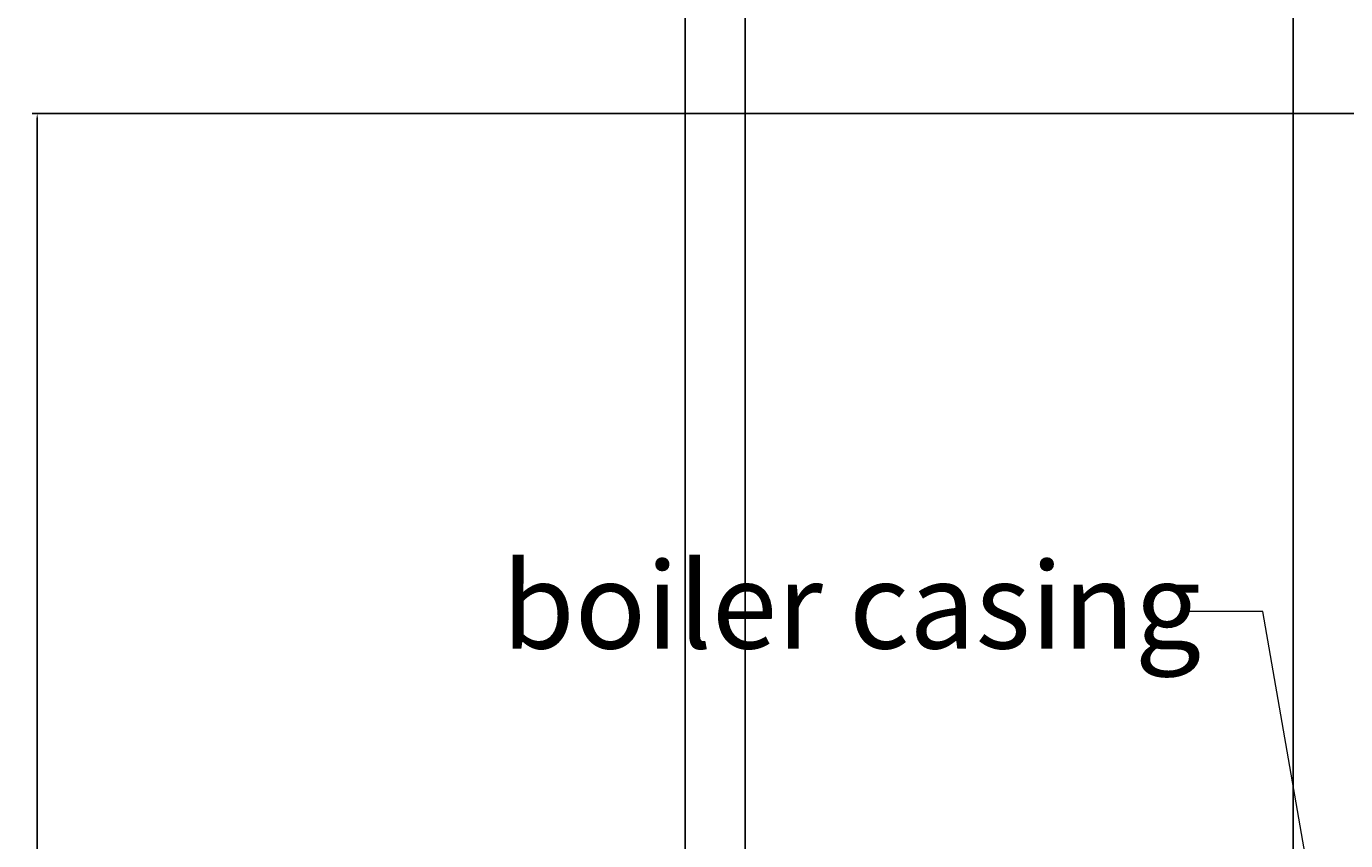
# Model space of a CAD drawing. Units: inches. Extents: x -1 to 292, y -3 to 199.
# Tile 11 of 52: x -1 to 45, y 101 to 130. Entities that reach past the tile are written whole.
import ezdxf

# ---------------------------------------------------------------- set-up
doc = ezdxf.new("R2010")
doc.units = ezdxf.units.IN
doc.header["$MEASUREMENT"] = 0
for name, color, linetype, lineweight in [('M-ANNO-LEAD', 2, 'Continuous', 18), ('M-ANNO-TEXT', 3, 'Continuous', 25), ('M-DIMS', 2, 'Continuous', 18)]:
    doc.layers.add(name, color=color, linetype=linetype, lineweight=lineweight)
doc.styles.get("Standard").update_dxf_attribs({"font": 'arial.ttf'})
doc.dimstyles.get("Standard").update_dxf_attribs({"dimtxt": 0.18, "dimasz": 0.18, "dimexe": 0.18, "dimexo": 0.0625, "dimgap": 0.09, "dimtad": 0, "dimtih": 1, "dimtoh": 1, "dimdec": 4, "dimzin": 0, "dimdsep": 46, "dimtxsty": 'Standard', "dimcen": 0.09, "dimadec": 0, "dimazin": 0, "dimtfac": 1, "dimtdec": 4, "dimtofl": 0, "dimtmove": 0, "dimatfit": 3, "dimfxl": 1, "dimtolj": 1, "dimtzin": 0, "dimarcsym": 0})

# ---------------------------------------------------------------- blocks, each defined once
blk = doc.blocks.new('*D8')
at = {"layer": 'Defpoints', "color": 0, "transparency": 16777216}
for p in [(-0.662, 126.765), (111.488, 126.765), (69.013, 25.514)]:
    blk.add_point(p, dxfattribs=at)
at = {"layer": 'M-DIMS', "color": 0, "lineweight": -2, "transparency": 16777216}
for p, q in [((111.426, 126.765), (-0.842, 126.765)), ((-0.662, 126.585), (-0.662, 76.321)), ((-0.662, 25.694), (-0.662, 75.958)), ((68.951, 25.514), (-0.842, 25.514))]:
    blk.add_line(p, q, dxfattribs=at)
at = {"layer": 'M-DIMS', "color": 0, "transparency": 16777216}
for points in [[(-0.692, 126.585), (-0.632, 126.585), (-0.662, 126.765)], [(-0.692, 25.694), (-0.632, 25.694), (-0.662, 25.514)]]:
    blk.add_solid(points, dxfattribs=at)
at = {"layer": 'M-DIMS', "color": 0, "transparency": 16777216, "insert": (-0.662, 76.14), "char_height": 0.18, "attachment_point": 5}
blk.add_mtext('\\A1;101.25', dxfattribs=at)
blk = doc.blocks.new('*D15')
at = {"layer": 'Defpoints', "color": 0, "transparency": 16777216}
for p in [(23.95, 174.363), (21.861, 88.582), (23.95, 88.582)]:
    blk.add_point(p, dxfattribs=at)
at = {"layer": 'M-DIMS', "color": 0, "lineweight": -2, "transparency": 16777216}
for p, q in [((21.861, 88.645), (21.861, 174.543)), ((22.041, 174.363), (22.51, 174.363)), ((23.77, 174.363), (23.301, 174.363)), ((23.95, 88.645), (23.95, 174.543))]:
    blk.add_line(p, q, dxfattribs=at)
at = {"layer": 'M-DIMS', "color": 0, "transparency": 16777216}
for points in [[(22.041, 174.393), (22.041, 174.333), (21.861, 174.363)], [(23.77, 174.393), (23.77, 174.333), (23.95, 174.363)]]:
    blk.add_solid(points, dxfattribs=at)
at = {"layer": 'M-DIMS', "color": 0, "transparency": 16777216, "insert": (22.906, 174.363), "char_height": 0.18, "attachment_point": 5}
blk.add_mtext('\\A1;2.089', dxfattribs=at)
blk = doc.blocks.new('*D16')
at = {"layer": 'Defpoints', "color": 0, "transparency": 16777216}
for p in [(42.998, 174.363), (42.998, 93.64), (23.95, 85.555)]:
    blk.add_point(p, dxfattribs=at)
at = {"layer": 'M-DIMS', "color": 0, "lineweight": -2, "transparency": 16777216}
for p, q in [((23.95, 85.618), (23.95, 174.543)), ((24.13, 174.363), (33.019, 174.363)), ((42.818, 174.363), (33.929, 174.363)), ((42.998, 93.703), (42.998, 174.543))]:
    blk.add_line(p, q, dxfattribs=at)
at = {"layer": 'M-DIMS', "color": 0, "transparency": 16777216}
for points in [[(24.13, 174.393), (24.13, 174.333), (23.95, 174.363)], [(42.818, 174.393), (42.818, 174.333), (42.998, 174.363)]]:
    blk.add_solid(points, dxfattribs=at)
at = {"layer": 'M-DIMS', "color": 0, "transparency": 16777216, "insert": (33.474, 174.363), "char_height": 0.18, "attachment_point": 5}
blk.add_mtext('\\A1;19.047', dxfattribs=at)

msp = doc.modelspace()

# ---------------------------------------------------------------- linework, layer by layer
at = {"layer": 'M-ANNO-LEAD'}
for p, q in [((41.954, 109.4627), (39.103, 109.4627)), ((44.6941, 93.6403), (41.954, 109.4627))]:
    msp.add_line(p, q, dxfattribs=at)

# ---------------------------------------------------------------- texts
at = {"layer": 'M-ANNO-TEXT', "insert": (15.4965, 111.1711), "char_height": 3, "attachment_point": 1}
msp.add_mtext_dynamic_manual_height_columns('boiler casing', width=47.899539, gutter_width=1, heights=[0], dxfattribs=at)

# ---------------------------------------------------------------- dimensions: what is measured, and where the dimension line sits
at = {"layer": 'M-DIMS'}
for base, p1, p2, picture, middle in [((23.9502, 174.3627), (21.8612, 88.5821), (23.9502, 88.5821), '*D15', (22.9057, 174.3627)), ((42.99769, 174.3627), (23.95023, 85.55517), (42.99769, 93.64034), '*D16', (33.47396, 174.3627))]:
    dim = msp.add_linear_dim(base=base, p1=p1, p2=p2, dimstyle='Standard', override={"dimdec": 3, "dimlfac": 1, "dimrnd": 0, "dimzin": 0, "dimdsep": 46, "dimlunit": 2}, dxfattribs=at)
    dim.commit()
    dim.dimension.update_dxf_attribs({"geometry": picture, "text_midpoint": middle})
dim = msp.add_linear_dim(base=(-0.6625, 126.765), p1=(69.013, 25.5141), p2=(111.4883, 126.765), angle=90, dimstyle='Standard', override={"dimdec": 2, "dimlfac": 1, "dimrnd": 0, "dimzin": 0, "dimdsep": 46, "dimlunit": 2}, dxfattribs=at)
dim.commit()
dim.dimension.update_dxf_attribs({"geometry": '*D8', "text_midpoint": (-0.6625, 76.1396)})

doc.saveas('drawing.dxf')
